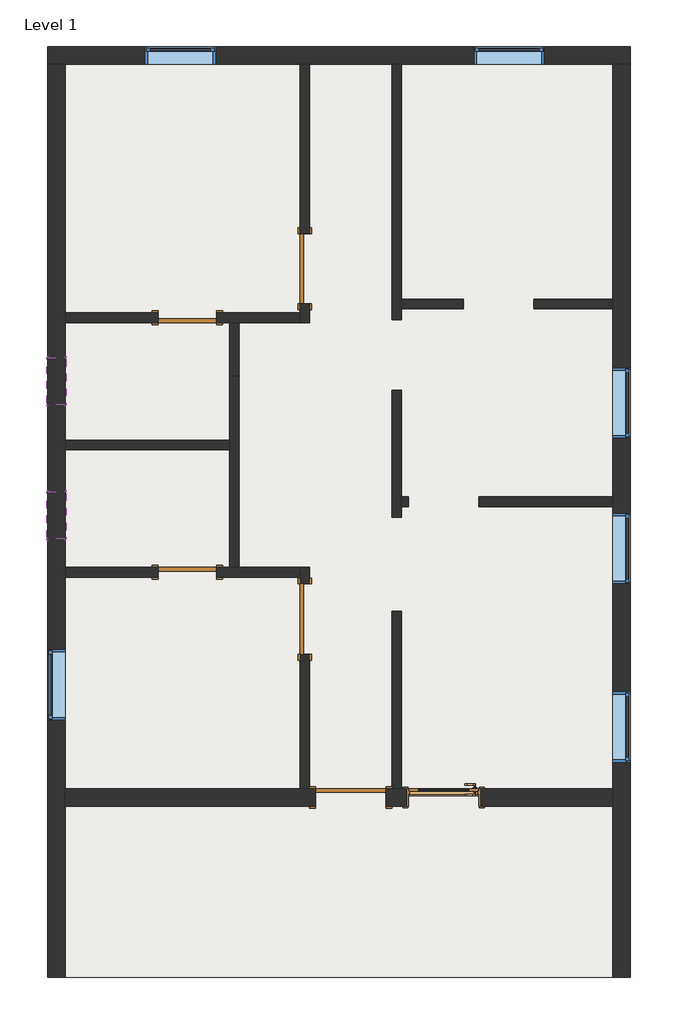
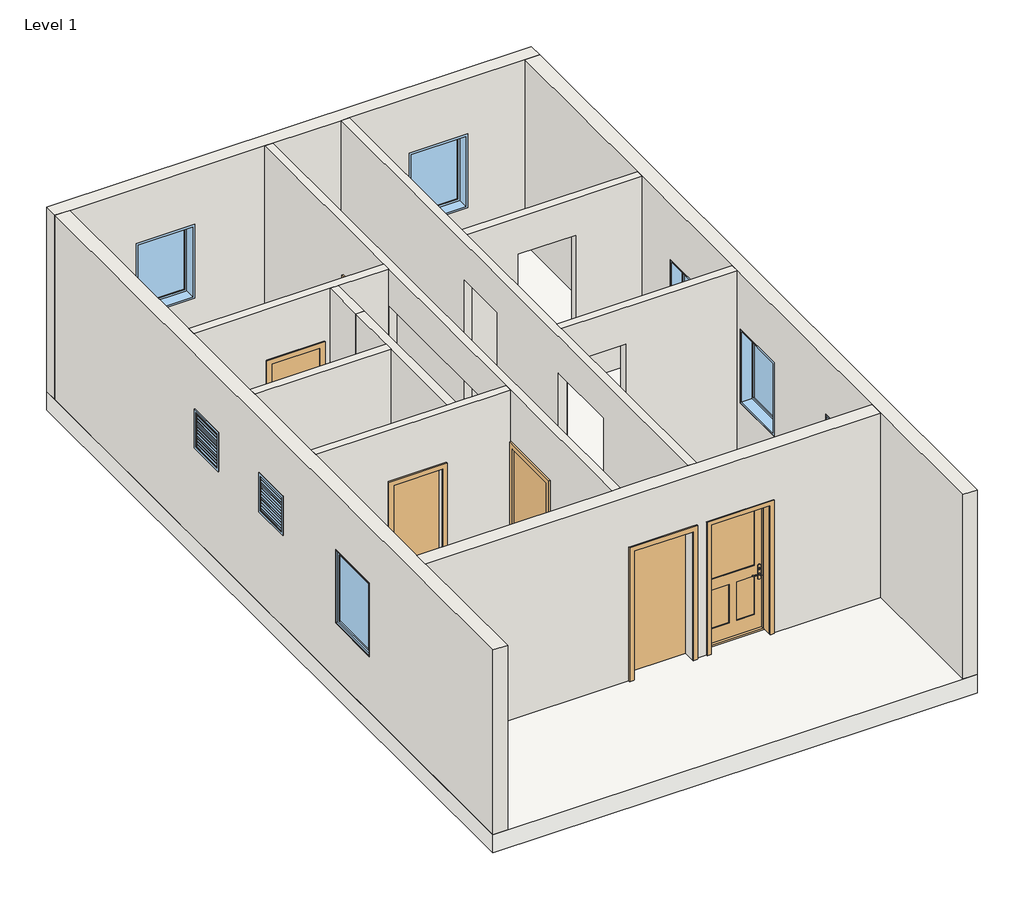
# One storey: 13 walls, 8 windows, 6 doors, 1 slab.
"""IFC4 building model written with IfcOpenShell, lengths in millimetres."""

from ifc_helpers import new_model, si_unit, frame, origin, origin_with_axes, place, context, project, spatial, polyline, outline, extrude, faceted_brep, transform, mapped, element, save
from components import door_16625766, door_4d6c7550, door_e36758a9, door_a3eb833a, door_a1797ceb, door_a90ba1ad, window_c1f32544, window_f2d8fef0

model = new_model("IFC4")

# Units and contexts
model_context = context("Model", 3, world=origin())
ifc_project = project(units=[si_unit("LENGTHUNIT", "METRE", prefix="MILLI")], contexts=[model_context])

# Site, building, storey
site = spatial("IfcSite", under=ifc_project)
building = spatial("IfcBuilding", under=site)
storey = spatial("IfcBuildingStorey", under=building, Name="Level 1", Elevation=0.0)

# Doors
placement = place(None, origin())
door_shape = door_16625766(model_context)
element("IfcDoor", 1, ObjectType="36\" x 84\"", at=placement, inside=storey, context=model_context, shape_type="MappedRepresentation", body=[
    mapped(door_shape, transform((-3233.05883, -2793.0844949, 0.0), x_axis=(1.0, 0.0, 0.0), y_axis=(0.0, 1.0, 0.0), z_axis=(0.0, 0.0, 1.0))),
])
door_2_shape = door_4d6c7550(model_context)
element("IfcDoor", 2, ObjectType="Single-Flush : 30\" x 84\"", at=placement, inside=storey, context=model_context, shape_type="MappedRepresentation", body=[
    mapped(door_2_shape, transform((-6560.45883, 124.7405051, 0.0), x_axis=(1.0, 0.0, 0.0), y_axis=(0.0, 1.0, 0.0), z_axis=(0.0, 0.0, 1.0))),
])
door_3_shape = door_e36758a9(model_context)
element("IfcDoor", 3, ObjectType="Single-Flush : 30\" x 84\"", at=placement, inside=storey, context=model_context, shape_type="MappedRepresentation", body=[
    mapped(door_3_shape, transform((-6560.45883, 3426.7405051, 0.0), x_axis=(1.0, 0.0, 0.0), y_axis=(0.0, 1.0, 0.0), z_axis=(0.0, 0.0, 1.0))),
])
door_4_shape = door_a3eb833a(model_context)
element("IfcDoor", 4, ObjectType="Single-Flush : 36\" x 84\"", at=placement, inside=storey, context=model_context, shape_type="MappedRepresentation", body=[
    mapped(door_4_shape, transform((-5036.45883, 4061.7405051, 0.0), x_axis=(0.0, -1.0, 0.0), y_axis=(1.0, 0.0, 0.0), z_axis=(0.0, 0.0, 1.0))),
])
door_5_shape = door_a1797ceb(model_context)
element("IfcDoor", 5, ObjectType="Single-Flush : 36\" x 84\"", at=placement, inside=storey, context=model_context, shape_type="MappedRepresentation", body=[
    mapped(door_5_shape, transform((-5036.45883, -484.8594949, 0.0), x_axis=(0.0, 1.0, 0.0), y_axis=(-1.0, 0.0, 0.0), z_axis=(0.0, 0.0, 1.0))),
])
door_6_shape = door_a90ba1ad(model_context)
element("IfcDoor", 6, ObjectType="Single-Flush : 36\" x 84\"", at=placement, inside=storey, context=model_context, shape_type="MappedRepresentation", body=[
    mapped(door_6_shape, transform((-4439.55883, -2796.2594949, 0.0), x_axis=(-1.0, 0.0, 0.0), y_axis=(0.0, -1.0, 0.0), z_axis=(0.0, 0.0, 1.0))),
])

# Slab
element("IfcSlab", 7, ObjectType="Generic - 12\"", at=placement, inside=storey, context=model_context, shape_type="SweptSolid", body=[
    extrude(outline(polyline([(-807.35883, 6944.6405051), (-807.35883, -5133.0594949), (-8376.55883, -5133.0594949), (-8376.55883, 6944.6405051), (-807.35883, 6944.6405051)])), frame((0.0, 0.0, -304.8), z_axis=(0.0, 0.0, 1.0), x_axis=(1.0, 0.0, 0.0)), (0.0, 0.0, 1.0), 304.8),
])

# Walls
element("IfcWall", 8, ObjectType="Generic - 5\"", at=placement, inside=storey, context=model_context, shape_type="Brep", body=[
    faceted_brep([(-5099.95883, 188.2405051, 0.0), (-5099.95883, 61.2405051, 0.0), (-5099.95883, -27.6594949, 0.0), (-5099.95883, -27.6594949, 2133.6), (-5099.95883, -942.0594949, 2133.6), (-5099.95883, -942.0594949, 0.0), (-5099.95883, -2681.9594949, 0.0), (-5099.95883, -2681.9594949, 3048.0), (-5099.95883, 61.2405051, 3048.0), (-5099.95883, 188.2405051, 3048.0), (-5099.95883, 3363.2405051, 3048.0), (-5099.95883, 3490.2405051, 3048.0), (-5099.95883, 6716.0405051, 3048.0), (-5099.95883, 6716.0405051, 0.0), (-5099.95883, 4518.9405051, 0.0), (-5099.95883, 4518.9405051, 2133.6), (-5099.95883, 3604.5405051, 2133.6), (-5099.95883, 3604.5405051, 0.0), (-5099.95883, 3490.2405051, 0.0), (-5099.95883, 3363.2405051, 0.0), (-5099.95883, 3363.2405051, 2438.4), (-5099.95883, 188.2405051, 2438.4), (-4972.95883, -27.6594949, 2133.6), (-4972.95883, -27.6594949, 0.0), (-4972.95883, 188.2405051, 0.0), (-4972.95883, 188.2405051, 2438.4), (-4972.95883, 3363.2405051, 2438.4), (-4972.95883, 3363.2405051, 0.0), (-4972.95883, 3604.5405051, 0.0), (-4972.95883, 3604.5405051, 2133.6), (-4972.95883, 4518.9405051, 2133.6), (-4972.95883, 4518.9405051, 0.0), (-4972.95883, 6716.0405051, 0.0), (-4972.95883, 6716.0405051, 3048.0), (-4972.95883, -2681.9594949, 3048.0), (-4972.95883, -2681.9594949, 0.0), (-4972.95883, -942.0594949, 0.0), (-4972.95883, -942.0594949, 2133.6)], [[[0, 1, 2, 3, 4, 5, 6, 7, 8, 9, 10, 11, 12, 13, 14, 15, 16, 17, 18, 19, 20, 21]], [[22, 23, 24, 25, 26, 27, 28, 29, 30, 31, 32, 33, 34, 35, 36, 37]], [[14, 13, 32, 31]], [[19, 18, 17, 28, 27]], [[36, 35, 6, 5]], [[24, 23, 2, 1, 0]], [[12, 11, 10, 9, 8, 7, 34, 33]], [[13, 12, 33, 32]], [[7, 6, 35, 34]], [[20, 26, 25, 21]], [[26, 20, 19, 27]], [[21, 25, 24, 0]], [[29, 28, 17, 16]], [[30, 29, 16, 15]], [[31, 30, 15, 14]], [[3, 2, 23, 22]], [[4, 3, 22, 37]], [[5, 4, 37, 36]]]),
])
element("IfcWall", 9, ObjectType="Generic - 5\"", at=placement, inside=storey, context=model_context, shape_type="Brep", body=[
    faceted_brep([(-3906.15883, -2681.9594949, 0.0), (-3906.15883, -2681.9594949, 3048.0), (-3906.15883, 6716.0405051, 3048.0), (-3906.15883, 6716.0405051, 0.0), (-3906.15883, 3401.3405051, 0.0), (-3906.15883, 3401.3405051, 2438.4), (-3906.15883, 2486.9405051, 2438.4), (-3906.15883, 2486.9405051, 0.0), (-3906.15883, 835.9405051, 0.0), (-3906.15883, 835.9405051, 2438.4), (-3906.15883, -383.2594949, 2438.4), (-3906.15883, -383.2594949, 0.0), (-3779.15883, -2681.9594949, 3048.0), (-3779.15883, -2681.9594949, 0.0), (-3779.15883, -383.2594949, 0.0), (-3779.15883, -383.2594949, 2438.4), (-3779.15883, 835.9405051, 2438.4), (-3779.15883, 835.9405051, 0.0), (-3779.15883, 975.6405051, 0.0), (-3779.15883, 1102.6405051, 0.0), (-3779.15883, 2486.9405051, 0.0), (-3779.15883, 2486.9405051, 2438.4), (-3779.15883, 3401.3405051, 2438.4), (-3779.15883, 3401.3405051, 0.0), (-3779.15883, 3541.0405051, 0.0), (-3779.15883, 3668.0405051, 0.0), (-3779.15883, 6716.0405051, 0.0), (-3779.15883, 6716.0405051, 3048.0), (-3779.15883, 3668.0405051, 3048.0), (-3779.15883, 3541.0405051, 3048.0), (-3779.15883, 1102.6405051, 3048.0), (-3779.15883, 975.6405051, 3048.0)], [[[0, 1, 2, 3, 4, 5, 6, 7, 8, 9, 10, 11]], [[12, 13, 14, 15, 16, 17, 18, 19, 20, 21, 22, 23, 24, 25, 26, 27, 28, 29, 30, 31]], [[3, 26, 25, 24, 23, 4]], [[13, 0, 11, 14]], [[7, 20, 19, 18, 17, 8]], [[2, 1, 12, 31, 30, 29, 28, 27]], [[3, 2, 27, 26]], [[1, 0, 13, 12]], [[5, 22, 21, 6]], [[22, 5, 4, 23]], [[6, 21, 20, 7]], [[9, 16, 15, 10]], [[16, 9, 8, 17]], [[10, 15, 14, 11]]]),
])
element("IfcWall", 10, ObjectType="Generic - 5\"", at=placement, inside=storey, context=model_context, shape_type="SweptSolid", body=[
    extrude(outline(polyline([(0.0, -1035.95883), (3048.0, -1035.95883), (3048.0, -3779.15883), (0.0, -3779.15883), (0.0, -2979.05883), (2438.4, -2979.05883), (2438.4, -2064.65883), (0.0, -2064.65883), (0.0, -1035.95883)])), frame((0.0, 3541.0405051, 0.0), z_axis=(0.0, 1.0, 0.0), x_axis=(0.0, 0.0, 1.0)), (0.0, 0.0, 1.0), 127.0),
])
element("IfcWall", 11, ObjectType="Generic - 5\"", at=placement, inside=storey, context=model_context, shape_type="SweptSolid", body=[
    extrude(outline(polyline([(0.0, -1035.95883), (3048.0, -1035.95883), (3048.0, -3779.15883), (0.0, -3779.15883), (0.0, -3690.25883), (2438.4, -3690.25883), (2438.4, -2775.85883), (0.0, -2775.85883), (0.0, -1035.95883)])), frame((0.0, 975.6405051, 0.0), z_axis=(0.0, 1.0, 0.0), x_axis=(0.0, 0.0, 1.0)), (0.0, 0.0, 1.0), 127.0),
])
element("IfcWall", 12, ObjectType="Generic - 5\"", at=placement, inside=storey, context=model_context, shape_type="Brep", body=[
    faceted_brep([(-5099.95883, 3490.2405051, 0.0), (-6179.45883, 3490.2405051, 0.0), (-6179.45883, 3490.2405051, 2133.6), (-6941.45883, 3490.2405051, 2133.6), (-6941.45883, 3490.2405051, 0.0), (-8147.95883, 3490.2405051, 0.0), (-8147.95883, 3490.2405051, 3048.0), (-5099.95883, 3490.2405051, 3048.0), (-6179.45883, 3363.2405051, 2133.6), (-6179.45883, 3363.2405051, 0.0), (-6014.35883, 3363.2405051, 0.0), (-5887.35883, 3363.2405051, 0.0), (-5099.95883, 3363.2405051, 0.0), (-5099.95883, 3363.2405051, 2438.4), (-5099.95883, 3363.2405051, 3048.0), (-5887.35883, 3363.2405051, 3048.0), (-6014.35883, 3363.2405051, 3048.0), (-8147.95883, 3363.2405051, 3048.0), (-8147.95883, 3363.2405051, 0.0), (-6941.45883, 3363.2405051, 0.0), (-6941.45883, 3363.2405051, 2133.6)], [[[0, 1, 2, 3, 4, 5, 6, 7]], [[8, 9, 10, 11, 12, 13, 14, 15, 16, 17, 18, 19, 20]], [[19, 18, 5, 4]], [[12, 11, 10, 9, 1, 0]], [[7, 6, 17, 16, 15, 14]], [[6, 5, 18, 17]], [[0, 7, 14, 13, 12]], [[2, 1, 9, 8]], [[3, 2, 8, 20]], [[4, 3, 20, 19]]]),
])
element("IfcWall", 13, ObjectType="Generic - 5\"", at=placement, inside=storey, context=model_context, shape_type="SweptSolid", body=[
    extrude(outline(polyline([(-6014.35883, 1712.2405051), (-8147.95883, 1712.2405051), (-8147.95883, 1839.2405051), (-6014.35883, 1839.2405051), (-6014.35883, 1712.2405051)])), origin_with_axes(), (0.0, 0.0, 1.0), 3048.0),
])
element("IfcWall", 14, ObjectType="Generic - 5\"", at=placement, inside=storey, context=model_context, shape_type="Brep", body=[
    faceted_brep([(-6179.45883, 61.2405051, 2133.6), (-6179.45883, 61.2405051, 0.0), (-5099.95883, 61.2405051, 0.0), (-5099.95883, 61.2405051, 3048.0), (-8147.95883, 61.2405051, 3048.0), (-8147.95883, 61.2405051, 0.0), (-6941.45883, 61.2405051, 0.0), (-6941.45883, 61.2405051, 2133.6), (-5099.95883, 188.2405051, 0.0), (-5887.35883, 188.2405051, 0.0), (-6014.35883, 188.2405051, 0.0), (-6179.45883, 188.2405051, 0.0), (-6179.45883, 188.2405051, 2133.6), (-6941.45883, 188.2405051, 2133.6), (-6941.45883, 188.2405051, 0.0), (-8147.95883, 188.2405051, 0.0), (-8147.95883, 188.2405051, 3048.0), (-6014.35883, 188.2405051, 3048.0), (-5887.35883, 188.2405051, 3048.0), (-5099.95883, 188.2405051, 3048.0), (-5099.95883, 188.2405051, 2438.4)], [[[0, 1, 2, 3, 4, 5, 6, 7]], [[8, 9, 10, 11, 12, 13, 14, 15, 16, 17, 18, 19, 20]], [[6, 5, 15, 14]], [[2, 1, 11, 10, 9, 8]], [[4, 3, 19, 18, 17, 16]], [[5, 4, 16, 15]], [[3, 2, 8, 20, 19]], [[12, 11, 1, 0]], [[13, 12, 0, 7]], [[14, 13, 7, 6]]]),
])
element("IfcWall", 15, ObjectType="Generic - 5\"", at=placement, inside=storey, context=model_context, shape_type="SweptSolid", body=[
    extrude(outline(polyline([(-5887.35883, 3363.2405051), (-5887.35883, 2664.7405051), (-6014.35883, 2664.7405051), (-6014.35883, 3363.2405051), (-5887.35883, 3363.2405051)])), origin_with_axes(), (0.0, 0.0, 1.0), 3048.0),
])
element("IfcWall", 16, ObjectType="Generic - 5\"", at=placement, inside=storey, context=model_context, shape_type="Brep", body=[
    faceted_brep([(-6014.35883, 2664.7405051, 0.0), (-6014.35883, 1839.2405051, 0.0), (-6014.35883, 1712.2405051, 0.0), (-6014.35883, 188.2405051, 0.0), (-6014.35883, 188.2405051, 3048.0), (-6014.35883, 1712.2405051, 3048.0), (-6014.35883, 1839.2405051, 3048.0), (-6014.35883, 2664.7405051, 3048.0), (-5887.35883, 2664.7405051, 0.0), (-5887.35883, 2664.7405051, 3048.0), (-5887.35883, 188.2405051, 3048.0), (-5887.35883, 188.2405051, 0.0)], [[[0, 1, 2, 3, 4, 5, 6, 7]], [[8, 9, 10, 11]], [[3, 2, 1, 0, 8, 11]], [[7, 6, 5, 4, 10, 9]], [[0, 7, 9, 8]], [[4, 3, 11, 10]]]),
])
element("IfcWall", 17, ObjectType="Generic - 9\"", at=placement, inside=storey, context=model_context, shape_type="Brep", body=[
    faceted_brep([(-8376.55883, 6716.0405051, 0.0), (-8147.95883, 6716.0405051, 0.0), (-5099.95883, 6716.0405051, 0.0), (-4972.95883, 6716.0405051, 0.0), (-3906.15883, 6716.0405051, 0.0), (-3779.15883, 6716.0405051, 0.0), (-1035.95883, 6716.0405051, 0.0), (-807.35883, 6716.0405051, 0.0), (-807.35883, 6716.0405051, 3048.0), (-1035.95883, 6716.0405051, 3048.0), (-3779.15883, 6716.0405051, 3048.0), (-3906.15883, 6716.0405051, 3048.0), (-4972.95883, 6716.0405051, 3048.0), (-5099.95883, 6716.0405051, 3048.0), (-8147.95883, 6716.0405051, 3048.0), (-8376.55883, 6716.0405051, 3048.0), (-6192.15883, 6716.0405051, 2133.6), (-6192.15883, 6716.0405051, 914.4), (-7106.55883, 6716.0405051, 914.4), (-7106.55883, 6716.0405051, 2133.6), (-1924.95883, 6716.0405051, 2133.6), (-1924.95883, 6716.0405051, 914.4), (-2839.35883, 6716.0405051, 914.4), (-2839.35883, 6716.0405051, 2133.6), (-8376.55883, 6944.6405051, 0.0), (-8376.55883, 6944.6405051, 3048.0), (-807.35883, 6944.6405051, 3048.0), (-807.35883, 6944.6405051, 0.0), (-6192.15883, 6944.6405051, 2133.6), (-7106.55883, 6944.6405051, 2133.6), (-7106.55883, 6944.6405051, 914.4), (-6192.15883, 6944.6405051, 914.4), (-1924.95883, 6944.6405051, 2133.6), (-2839.35883, 6944.6405051, 2133.6), (-2839.35883, 6944.6405051, 914.4), (-1924.95883, 6944.6405051, 914.4)], [[[0, 1, 2, 3, 4, 5, 6, 7, 8, 9, 10, 11, 12, 13, 14, 15], [16, 17, 18, 19], [20, 21, 22, 23]], [[24, 25, 26, 27], [28, 29, 30, 31], [32, 33, 34, 35]], [[7, 6, 5, 4, 3, 2, 1, 0, 24, 27]], [[15, 14, 13, 12, 11, 10, 9, 8, 26, 25]], [[8, 7, 27, 26]], [[0, 15, 25, 24]], [[17, 16, 28, 31]], [[18, 17, 31, 30]], [[19, 18, 30, 29]], [[16, 19, 29, 28]], [[21, 20, 32, 35]], [[22, 21, 35, 34]], [[23, 22, 34, 33]], [[20, 23, 33, 32]]]),
])
element("IfcWall", 18, ObjectType="Generic - 9\"", at=placement, inside=storey, context=model_context, shape_type="Brep", body=[
    faceted_brep([(-1035.95883, 6716.0405051, 0.0), (-1035.95883, 3668.0405051, 0.0), (-1035.95883, 3541.0405051, 0.0), (-1035.95883, 1102.6405051, 0.0), (-1035.95883, 975.6405051, 0.0), (-1035.95883, -2681.9594949, 0.0), (-1035.95883, -2910.5594949, 0.0), (-1035.95883, -5133.0594949, 0.0), (-1035.95883, -5133.0594949, 3048.0), (-1035.95883, -2910.5594949, 3048.0), (-1035.95883, -2681.9594949, 3048.0), (-1035.95883, 975.6405051, 3048.0), (-1035.95883, 1102.6405051, 3048.0), (-1035.95883, 3541.0405051, 3048.0), (-1035.95883, 3668.0405051, 3048.0), (-1035.95883, 6716.0405051, 3048.0), (-1035.95883, -2339.0594949, 2133.6), (-1035.95883, -2339.0594949, 914.4), (-1035.95883, -1424.6594949, 914.4), (-1035.95883, -1424.6594949, 2133.6), (-1035.95883, -27.6594949, 2133.6), (-1035.95883, -27.6594949, 914.4), (-1035.95883, 886.7405051, 914.4), (-1035.95883, 886.7405051, 2133.6), (-1035.95883, 1864.6405051, 2133.6), (-1035.95883, 1864.6405051, 914.4), (-1035.95883, 2779.0405051, 914.4), (-1035.95883, 2779.0405051, 2133.6), (-807.35883, 6716.0405051, 0.0), (-807.35883, 6716.0405051, 3048.0), (-807.35883, -5133.0594949, 3048.0), (-807.35883, -5133.0594949, 0.0), (-807.35883, -2339.0594949, 2133.6), (-807.35883, -1424.6594949, 2133.6), (-807.35883, -1424.6594949, 914.4), (-807.35883, -2339.0594949, 914.4), (-807.35883, -27.6594949, 2133.6), (-807.35883, 886.7405051, 2133.6), (-807.35883, 886.7405051, 914.4), (-807.35883, -27.6594949, 914.4), (-807.35883, 1864.6405051, 2133.6), (-807.35883, 2779.0405051, 2133.6), (-807.35883, 2779.0405051, 914.4), (-807.35883, 1864.6405051, 914.4)], [[[0, 1, 2, 3, 4, 5, 6, 7, 8, 9, 10, 11, 12, 13, 14, 15], [16, 17, 18, 19], [20, 21, 22, 23], [24, 25, 26, 27]], [[28, 29, 30, 31], [32, 33, 34, 35], [36, 37, 38, 39], [40, 41, 42, 43]], [[7, 6, 5, 4, 3, 2, 1, 0, 28, 31]], [[8, 7, 31, 30]], [[15, 14, 13, 12, 11, 10, 9, 8, 30, 29]], [[0, 15, 29, 28]], [[17, 16, 32, 35]], [[18, 17, 35, 34]], [[19, 18, 34, 33]], [[16, 19, 33, 32]], [[21, 20, 36, 39]], [[22, 21, 39, 38]], [[23, 22, 38, 37]], [[20, 23, 37, 36]], [[25, 24, 40, 43]], [[26, 25, 43, 42]], [[27, 26, 42, 41]], [[24, 27, 41, 40]]]),
])
element("IfcWall", 19, ObjectType="Generic - 9\"", at=placement, inside=storey, context=model_context, shape_type="Brep", body=[
    faceted_brep([(-8147.95883, -5133.0594949, 0.0), (-8147.95883, -2910.5594949, 0.0), (-8147.95883, -2681.9594949, 0.0), (-8147.95883, 61.2405051, 0.0), (-8147.95883, 188.2405051, 0.0), (-8147.95883, 1712.2405051, 0.0), (-8147.95883, 1839.2405051, 0.0), (-8147.95883, 3363.2405051, 0.0), (-8147.95883, 3490.2405051, 0.0), (-8147.95883, 6716.0405051, 0.0), (-8147.95883, 6716.0405051, 3048.0), (-8147.95883, 3490.2405051, 3048.0), (-8147.95883, 3363.2405051, 3048.0), (-8147.95883, 1839.2405051, 3048.0), (-8147.95883, 1712.2405051, 3048.0), (-8147.95883, 188.2405051, 3048.0), (-8147.95883, 61.2405051, 3048.0), (-8147.95883, -2681.9594949, 3048.0), (-8147.95883, -2910.5594949, 3048.0), (-8147.95883, -5133.0594949, 3048.0), (-8147.95883, -878.5594949, 2133.6), (-8147.95883, -878.5594949, 914.4), (-8147.95883, -1792.9594949, 914.4), (-8147.95883, -1792.9594949, 2133.6), (-8147.95883, 2296.4405051, 2133.6), (-8147.95883, 2906.0405051, 2133.6), (-8147.95883, 2906.0405051, 1524.0), (-8147.95883, 2296.4405051, 1524.0), (-8147.95883, 556.5405051, 2133.6), (-8147.95883, 1166.1405051, 2133.6), (-8147.95883, 1166.1405051, 1524.0), (-8147.95883, 556.5405051, 1524.0), (-8376.55883, -5133.0594949, 0.0), (-8376.55883, -5133.0594949, 3048.0), (-8376.55883, 6716.0405051, 3048.0), (-8376.55883, 6716.0405051, 0.0), (-8376.55883, -878.5594949, 2133.6), (-8376.55883, -1792.9594949, 2133.6), (-8376.55883, -1792.9594949, 914.4), (-8376.55883, -878.5594949, 914.4), (-8376.55883, 2296.4405051, 2133.6), (-8376.55883, 2296.4405051, 1524.0), (-8376.55883, 2906.0405051, 1524.0), (-8376.55883, 2906.0405051, 2133.6), (-8376.55883, 556.5405051, 2133.6), (-8376.55883, 556.5405051, 1524.0), (-8376.55883, 1166.1405051, 1524.0), (-8376.55883, 1166.1405051, 2133.6)], [[[0, 1, 2, 3, 4, 5, 6, 7, 8, 9, 10, 11, 12, 13, 14, 15, 16, 17, 18, 19], [20, 21, 22, 23], [24, 25, 26, 27], [28, 29, 30, 31]], [[32, 33, 34, 35], [36, 37, 38, 39], [40, 41, 42, 43], [44, 45, 46, 47]], [[9, 8, 7, 6, 5, 4, 3, 2, 1, 0, 32, 35]], [[19, 18, 17, 16, 15, 14, 13, 12, 11, 10, 34, 33]], [[0, 19, 33, 32]], [[10, 9, 35, 34]], [[21, 20, 36, 39]], [[22, 21, 39, 38]], [[23, 22, 38, 37]], [[20, 23, 37, 36]], [[41, 40, 24, 27]], [[42, 41, 27, 26]], [[43, 42, 26, 25]], [[40, 43, 25, 24]], [[45, 44, 28, 31]], [[46, 45, 31, 30]], [[47, 46, 30, 29]], [[44, 47, 29, 28]]]),
])
element("IfcWall", 20, ObjectType="Generic - 9\"", at=placement, inside=storey, context=model_context, shape_type="Brep", body=[
    faceted_brep([(-1035.95883, -2910.5594949, 3048.0), (-8147.95883, -2910.5594949, 3048.0), (-8147.95883, -2910.5594949, 0.0), (-4896.75883, -2910.5594949, 0.0), (-4896.75883, -2910.5594949, 2133.6), (-3982.35883, -2910.5594949, 2133.6), (-3982.35883, -2910.5594949, 0.0), (-3715.65883, -2910.5594949, 0.0), (-3715.65883, -2910.5594949, 2159.0), (-2750.45883, -2910.5594949, 2159.0), (-2750.45883, -2910.5594949, 0.0), (-1035.95883, -2910.5594949, 0.0), (-8147.95883, -2681.9594949, 3048.0), (-5099.95883, -2681.9594949, 3048.0), (-4972.95883, -2681.9594949, 3048.0), (-3906.15883, -2681.9594949, 3048.0), (-3779.15883, -2681.9594949, 3048.0), (-1035.95883, -2681.9594949, 3048.0), (-1035.95883, -2681.9594949, 0.0), (-2750.45883, -2681.9594949, 0.0), (-2750.45883, -2681.9594949, 2159.0), (-3715.65883, -2681.9594949, 2159.0), (-3715.65883, -2681.9594949, 0.0), (-3779.15883, -2681.9594949, 0.0), (-3906.15883, -2681.9594949, 0.0), (-3982.35883, -2681.9594949, 0.0), (-3982.35883, -2681.9594949, 2133.6), (-4896.75883, -2681.9594949, 2133.6), (-4896.75883, -2681.9594949, 0.0), (-4972.95883, -2681.9594949, 0.0), (-5099.95883, -2681.9594949, 0.0), (-8147.95883, -2681.9594949, 0.0)], [[[0, 1, 2, 3, 4, 5, 6, 7, 8, 9, 10, 11]], [[12, 13, 14, 15, 16, 17, 18, 19, 20, 21, 22, 23, 24, 25, 26, 27, 28, 29, 30, 31]], [[18, 11, 10, 19]], [[2, 31, 30, 29, 28, 3]], [[6, 25, 24, 23, 22, 7]], [[1, 0, 17, 16, 15, 14, 13, 12]], [[0, 11, 18, 17]], [[2, 1, 12, 31]], [[4, 3, 28, 27]], [[5, 4, 27, 26]], [[6, 5, 26, 25]], [[9, 20, 19, 10]], [[20, 9, 8, 21]], [[21, 8, 7, 22]]]),
])

# Windows
window_shape = window_c1f32544(model_context)
element("IfcWindow", 21, ObjectType="Fixed : 36\" x 48\"", at=placement, inside=storey, context=model_context, shape_type="MappedRepresentation", body=[
    mapped(window_shape, transform((-6611.25883, 6830.3405051, 0.0), x_axis=(1.0, 0.0, 0.0), y_axis=(0.0, 1.0, 0.0), z_axis=(0.0, 0.0, 1.0))),
])
element("IfcWindow", 22, ObjectType="Fixed : 36\" x 48\"", at=placement, inside=storey, context=model_context, shape_type="MappedRepresentation", body=[
    mapped(window_shape, transform((-2344.05883, 6830.3405051, 0.0), x_axis=(1.0, 0.0, 0.0), y_axis=(0.0, 1.0, 0.0), z_axis=(0.0, 0.0, 1.0))),
])
element("IfcWindow", 23, ObjectType="Fixed : 36\" x 48\"", at=placement, inside=storey, context=model_context, shape_type="MappedRepresentation", body=[
    mapped(window_shape, transform((-8262.25883, -1297.6594949, 0.0), x_axis=(0.0, 1.0, 0.0), y_axis=(-1.0, 0.0, 0.0), z_axis=(0.0, 0.0, 1.0))),
])
element("IfcWindow", 24, ObjectType="Fixed : 36\" x 48\"", at=placement, inside=storey, context=model_context, shape_type="MappedRepresentation", body=[
    mapped(window_shape, transform((-921.65883, -1919.9594949, 0.0), x_axis=(0.0, -1.0, 0.0), y_axis=(1.0, 0.0, 0.0), z_axis=(0.0, 0.0, 1.0))),
])
element("IfcWindow", 25, ObjectType="Fixed : 36\" x 48\"", at=placement, inside=storey, context=model_context, shape_type="MappedRepresentation", body=[
    mapped(window_shape, transform((-921.65883, 391.4405051, 0.0), x_axis=(0.0, -1.0, 0.0), y_axis=(1.0, 0.0, 0.0), z_axis=(0.0, 0.0, 1.0))),
])
element("IfcWindow", 26, ObjectType="Fixed : 36\" x 48\"", at=placement, inside=storey, context=model_context, shape_type="MappedRepresentation", body=[
    mapped(window_shape, transform((-921.65883, 2283.7405051, 0.0), x_axis=(0.0, -1.0, 0.0), y_axis=(1.0, 0.0, 0.0), z_axis=(0.0, 0.0, 1.0))),
])
window_2_shape = window_f2d8fef0(model_context)
element("IfcWindow", 27, ObjectType="Window-Louvers : 24\" x 24\"", at=placement, inside=storey, context=model_context, shape_type="MappedRepresentation", body=[
    mapped(window_2_shape, transform((-8268.60883, 2601.2405051, 609.6), x_axis=(0.0, 1.0, 0.0), y_axis=(-1.0, 0.0, 0.0), z_axis=(0.0, 0.0, 1.0))),
])
element("IfcWindow", 28, ObjectType="Window-Louvers : 24\" x 24\"", at=placement, inside=storey, context=model_context, shape_type="MappedRepresentation", body=[
    mapped(window_2_shape, transform((-8268.60883, 861.3405051, 609.6), x_axis=(0.0, 1.0, 0.0), y_axis=(-1.0, 0.0, 0.0), z_axis=(0.0, 0.0, 1.0))),
])

save(model, "model.ifc")

# Revit data of these elements
# Type "36\" x 84\""
#   Type Mark = "8"
#   Assembly Code = "B2030100"
#   Analytic Construction = "French door, wood frame with single glass"
#   Top Rail = 0' - 4 3/4"
#   Threshold Offset [instance default] = 0' - 0 1/2"
#   Thickness = 0' - 1 3/8"
#   Thermal Resistance (R) = 1.0696 (h·ft²·°F)/BTU
#   Swing Angle [instance default] = 90.00°
#   Stiles = 0' - 4 3/4"
#   Rough Width = 3' - 2"
#   Rough Height = 7' - 1"
#   Lock Rail = 0' - 7 1/8"
#   Height = 7' - 0"
#   Width = 3' - 0"
#   Heat Transfer Coefficient (U) = 0.9350 BTU/(h·ft²·°F)
#   Door Offset [instance default] = 0' - 0"
#   Bottom Rail = 0' - 9 1/2"
#   Threshold [instance default] = yes
#   Function = 1
#   Exterior Trim [instance default] = yes
#   Trim Material = Cherry
#   Threshold Material = Cherry
#   Panel Material = Cherry
#   Glazing = Glass
#   Frame Material = Cherry
#   Door Handle Material = Aluminum
#   Visual Light Transmittance = 0
#   Solar Heat Gain Coefficient = 0
#   Wall Closure = (empty or 0)
#   Construction Type = (empty or 0)
# Type "Single-Flush : 30\" x 84\""
#   Type Mark = "4"
#   Construction Type Id = "MDOOR"
#   Assembly Code = "C1020"
#   Analytic Construction = "Metal"
#   Thickness = 0' - 2"
#   Heat Transfer Coefficient (U) = 0.651978 BTU/(h·ft²·°F)
#   Height = 7' - 0"
#   Trim Projection Ext = 0' - 1"
#   Trim Projection Int = 0' - 1"
#   Trim Width = 0' - 3"
#   Width = 2' - 6"
#   Define Thermal Properties by = 1
#   Define Thermal Properties by = 1
#   Door Material = Door - Panel
#   Frame Material = Door - Frame
#   Visual Light Transmittance = 0
#   Solar Heat Gain Coefficient = 0
#   Function = (empty or 0)
#   Wall Closure = (empty or 0)
# Type "Single-Flush : 36\" x 84\""
#   Type Mark = "1"
#   Construction Type Id = "MDOOR"
#   Assembly Code = "C1020"
#   Analytic Construction = "Metal"
#   Thickness = 0' - 2"
#   Heat Transfer Coefficient (U) = 0.651978 BTU/(h·ft²·°F)
#   Height = 7' - 0"
#   Trim Projection Ext = 0' - 1"
#   Trim Projection Int = 0' - 1"
#   Trim Width = 0' - 3"
#   Width = 3' - 0"
#   Define Thermal Properties by = 1
#   Define Thermal Properties by = 1
#   Door Material = Door - Panel
#   Frame Material = Door - Frame
#   Visual Light Transmittance = 0
#   Solar Heat Gain Coefficient = 0
#   Function = (empty or 0)
#   Wall Closure = (empty or 0)
# Type "Generic - 12\""
#   Assembly Code = "B1010"
#   Function = 0
#   Layers, outside or top first: 1' - 0" no material (function 1)
# Type "Generic - 5\""
#   Assembly Code = "B2010"
#   Layers, outside or top first: 0' - 5" no material (function 1)
# Type "Generic - 9\""
#   Assembly Code = "B2010"
#   Layers, outside or top first: 0' - 9" no material (function 1)
# Type "Fixed : 36\" x 48\""
#   Type Mark = "1"
#   Construction Type Id = "GSP4R"
#   Assembly Code = "B2020100"
#   Analytic Construction = "1/8 in Pilkington single glazing"
#   Visual Light Transmittance = 0.9
#   Solar Heat Gain Coefficient = 0.78
#   Heat Transfer Coefficient (U) = 0.6496 BTU/(h·ft²·°F)
#   Height = 4' - 0"
#   Default Sill Height = 3' - 0"
#   Width = 3' - 0"
#   Window Inset = 0' - 0 3/4"
#   Define Thermal Properties by = 1
#   Define Thermal Properties by = 1
#   Glass Pane Material = Glass
#   Sash Material = Sash
#   Wall Closure = (empty or 0)
# Type "Window-Louvers : 24\" x 24\""
#   Type Mark = "18"
#   Construction Type Id = "GSP4R"
#   Assembly Code = "B20"
#   Analytic Construction = "1/8 in Pilkington single glazing"
#   Visual Light Transmittance = 0.9
#   Thermal Resistance (R) = 1.53941 (h·ft²·°F)/BTU
#   Solar Heat Gain Coefficient = 0.78
#   Max Height = 1' - 11.74264"
#   Height = 2' - 0"
#   Heat Transfer Coefficient (U) = 0.6496 BTU/(h·ft²·°F)
#   Blade Width [instance default] = 1' - 10 1/2"
#   Blade Vertical Thickness = 0' - 0.35355"
#   Blade Thickness = 0' - 0 1/4"
#   Blade Spacing = 0' - 1 1/2"
#   Blade Height = 0' - 1.85355"
#   Blade Depth = 0' - 3"
#   Blade Angle = 45.00°
#   Default Sill Height = 3' - 0"
#   Trim Projection_Exterior = 0' - 0 1/2"
#   Trim Projection_Interior = 0' - 0 1/2"
#   Trim Width_Exterior = 0' - 1 1/2"
#   Trim Width_Interior = 0' - 1 1/2"
#   Width = 2' - 0"
#   Max Blade Count = 12
#   Define Thermal Properties by = 1
#   Blade Count = 12
#   Frame Material = Birch
#   Louver Material = Birch
#   Trim Exterior Material = Birch
#   Trim Interior Material = Birch
#   Wall Closure = (empty or 0)
# Element 1 (IfcDoor, "36\" x 84\"")
#   Threshold Offset = 0' - 0 1/2"
#   Swing Angle = 90.00°
#   Door Offset = 0' - 0"
#   Threshold = yes
#   Exterior Trim = yes
#   Phase Created = New Construction
#   Materials on its faces: "Cherry", "Aluminum", "Glass"
# Elements 2, 3 (IfcDoor, "Single-Flush : 30\" x 84\"")
#   Phase Created = New Construction
#   Materials on its faces: "Door - Frame", "Door - Panel"
# Elements 4, 5, 6 (IfcDoor, "Single-Flush : 36\" x 84\"")
#   Phase Created = New Construction
#   Materials on its faces: "Door - Frame", "Door - Panel"
# Element 7 (IfcSlab, "Generic - 12\"")
#   Height Offset From Level = 0' - 0"
#   Phase Created = New Construction
#   Materials on its faces: "Default Floor"
# Elements 8, 9, 10, 11, 12, 13, 14, 15, 16 (IfcWall, "Generic - 5\"")
#   Top Offset = 0' - 0"
#   Base Offset = 0' - 0"
#   wall height = 10' - 0"
#   Phase Created = New Construction
#   Base Constraint = Level 1
#   Top Constraint = Level 2
#   Materials on its faces: "Default Wall"
# Elements 17, 18, 19, 20 (IfcWall, "Generic - 9\"")
#   Top Offset = 0' - 0"
#   Base Offset = 0' - 0"
#   wall height = 10' - 0"
#   Phase Created = New Construction
#   Base Constraint = Level 1
#   Top Constraint = Level 2
#   Materials on its faces: "Default Wall"
# Element 21 (IfcWindow, "Fixed : 36\" x 48\"")
#   Mark = "1"
#   Phase Created = New Construction
#   Materials on its faces: "Sash", "Glass"
# Element 22 (IfcWindow, "Fixed : 36\" x 48\"")
#   Mark = "2"
#   Phase Created = New Construction
#   Materials on its faces: "Sash", "Glass"
# Element 23 (IfcWindow, "Fixed : 36\" x 48\"")
#   Mark = "3"
#   Phase Created = New Construction
#   Materials on its faces: "Sash", "Glass"
# Element 24 (IfcWindow, "Fixed : 36\" x 48\"")
#   Mark = "4"
#   Phase Created = New Construction
#   Materials on its faces: "Sash", "Glass"
# Element 25 (IfcWindow, "Fixed : 36\" x 48\"")
#   Mark = "5"
#   Phase Created = New Construction
#   Materials on its faces: "Sash", "Glass"
# Element 26 (IfcWindow, "Fixed : 36\" x 48\"")
#   Mark = "6"
#   Phase Created = New Construction
#   Materials on its faces: "Sash", "Glass"
# Element 27 (IfcWindow, "Window-Louvers : 24\" x 24\"")
#   Mark = "7"
#   Blade Width = 1' - 10 1/2"
#   Phase Created = New Construction
#   Materials on its faces: "Birch"
# Element 28 (IfcWindow, "Window-Louvers : 24\" x 24\"")
#   Mark = "8"
#   Blade Width = 1' - 10 1/2"
#   Phase Created = New Construction
#   Materials on its faces: "Birch"
# Materials
#   "Cherry": class "Wood", colour RGB 226 177 128, transparency 0, Description = "Prunus Serotina", Cost = 0
#   "Glass": class "Glass", colour RGB 0 128 192, transparency 0.75, Description = "Soda Lime Glass", Cost = 0
#   "Aluminum": class "Metal", colour RGB 247 247 247, transparency 0, Description = "Aluminum 6061", Cost = 0
#   "Door - Panel": class "Wood", colour RGB 210 159 95, transparency 0, Cost = 0
#   "Door - Frame": colour RGB 118 70 51, transparency 0, Cost = 0
#   "Sash": class "Wood", colour RGB 224 178 126, transparency 0, Cost = 0
#   "Birch": class "Wood", colour RGB 224 178 126, transparency 0, Description = "Betula Alleghaniensis", Cost = 0
#   "Default Floor": colour RGB 128 128 128, transparency 0, Cost = 0
#   "Default Wall": colour RGB 128 128 128, transparency 0, Cost = 0
# Room at (-6478.919, 5409.285) mm, phase "New Construction", upper level "Level 1", upper offset 10' - 0", lower offset 0' - 0"
#   Number = "10'X11'"
#   Name = "BEDROOM 1"
# Room at (-2276.883, 5150.698) mm, phase "New Construction", upper level "Level 1", upper offset 10' - 0", lower offset 0' - 0"
#   Number = "9'X10'"
#   Name = "KITCHEN"
# Room at (-2548.399, 2138.161) mm, phase "New Construction", upper level "Level 1", upper offset 10' - 0", lower offset 0' - 0"
#   Number = "9'X8'"
#   Name = "DINING"
# Room at (-2276.883, -874.179) mm, phase "New Construction", upper level "Level 1", upper offset 10' - 0", lower offset 0' - 0"
#   Number = "12'X12'"
#   Name = "LIVING ROOM"
# Room at (-6478.919, -1275.635) mm, phase "New Construction", upper level "Level 1", upper offset 10' - 0", lower offset 0' - 0"
#   Number = "5"
#   Name = "BED ROOM 2"
# Room at (-6896.394, 1147.97) mm, phase "New Construction", upper level "Level 1", upper offset 10' - 0", lower offset 0' - 0"
#   Number = "5'X7'"
#   Name = "BATH 2"
# Room at (-6896.394, 2407.162) mm, phase "New Construction", upper level "Level 1", upper offset 10' - 0", lower offset 0' - 0"
#   Number = "5'X7'"
#   Name = "BATH 1"
# Room at (-4650.119, 1636.618) mm, phase "New Construction", upper level "Level 1", upper offset 10' - 0", lower offset 0' - 0"
#   Number = "8"
#   Name = "PASSAGE"
